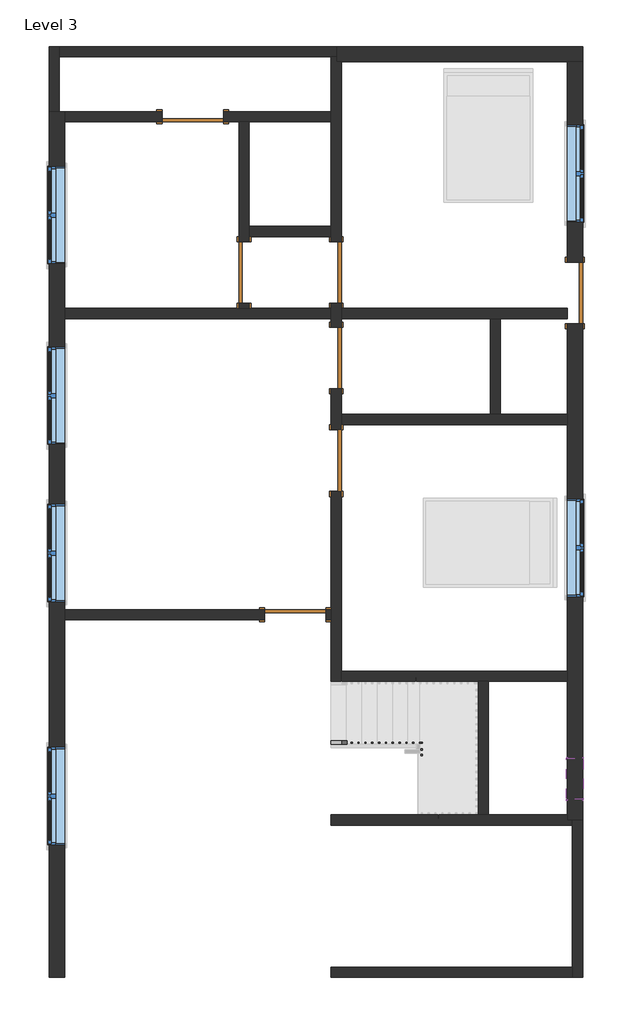
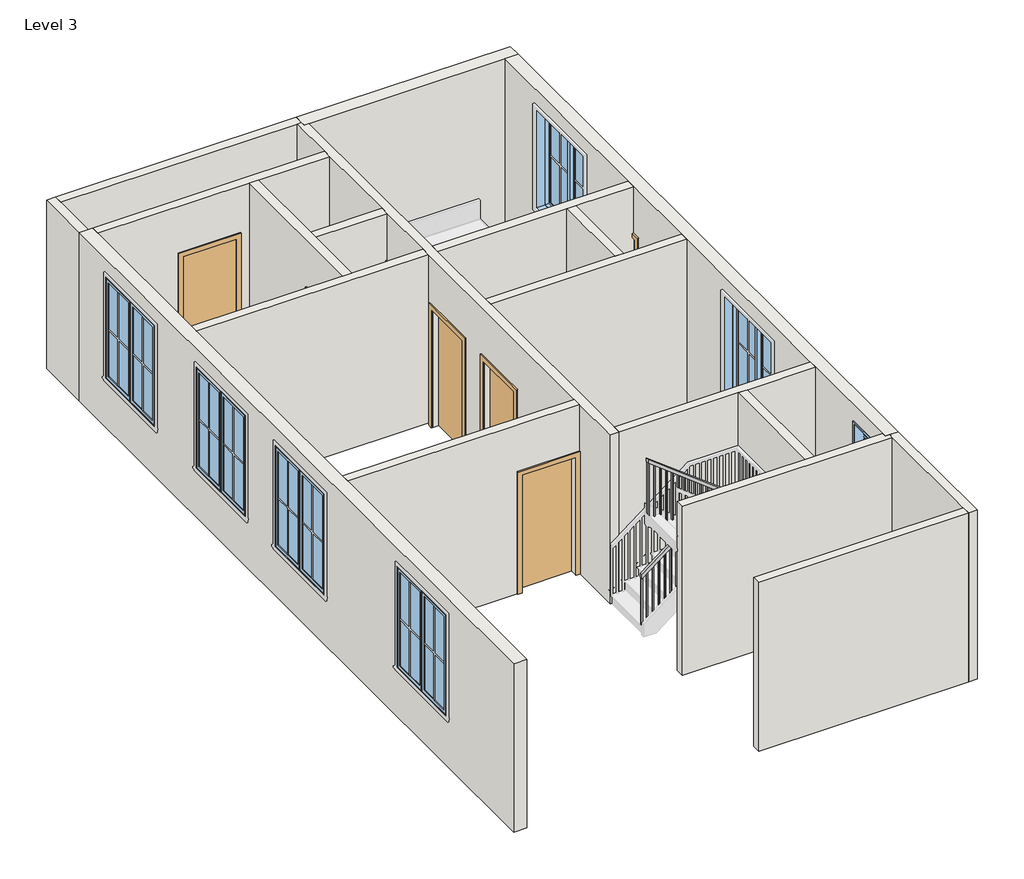
# One storey, part 1 of 2: 18 walls, 7 doors, 7 windows, 1 railing.
"""IFC4 building model written with IfcOpenShell, lengths in millimetres."""

from ifc_helpers import new_model, si_unit, frame, origin, place, context, project, spatial, polyline, outline, extrude, faceted_brep, transform, mapped, element, save
from components import door_686f89d2, door_16372e1c, door_0ca8825f, window_9ac97e1a, window_f2d8fef0

model = new_model("IFC4")

# Units and contexts
model_context = context("Model", 3, world=origin())
ifc_project = project(units=[si_unit("LENGTHUNIT", "METRE", prefix="MILLI")], contexts=[model_context])

# Site, building, storey
site = spatial("IfcSite", under=ifc_project)
building = spatial("IfcBuilding", under=site)
storey = spatial("IfcBuildingStorey", under=building, Name="Level 3", Elevation=3200.4)

# Doors
placement = place(None, origin())
door_shape = door_686f89d2(model_context)
element("IfcDoor", 1, ObjectType="Single-Flush : 36\" x 84\"", at=placement, inside=storey, context=model_context, shape_type="MappedRepresentation", body=[
    mapped(door_shape, transform((-2318.0415352, 3143.9226491, 3200.4), x_axis=(0.0, -1.0, 0.0), y_axis=(1.0, 0.0, 0.0), z_axis=(0.0, 0.0, 1.0))),
])
element("IfcDoor", 2, ObjectType="Single-Flush : 36\" x 84\"", at=placement, inside=storey, context=model_context, shape_type="MappedRepresentation", body=[
    mapped(door_shape, transform((-946.4415352, 3143.7222669, 3200.4), x_axis=(0.0, 1.0, 0.0), y_axis=(-1.0, 0.0, 0.0), z_axis=(0.0, 0.0, 1.0))),
])
element("IfcDoor", 3, ObjectType="Single-Flush : 36\" x 84\"", at=placement, inside=storey, context=model_context, shape_type="MappedRepresentation", body=[
    mapped(door_shape, transform((-946.4415352, 1874.1230313, 3200.4), x_axis=(0.0, 1.0, 0.0), y_axis=(-1.0, 0.0, 0.0), z_axis=(0.0, 0.0, 1.0))),
])
element("IfcDoor", 4, ObjectType="Single-Flush : 36\" x 84\"", at=placement, inside=storey, context=model_context, shape_type="MappedRepresentation", body=[
    mapped(door_shape, transform((-946.4415352, 350.1230313, 3200.4), x_axis=(0.0, 1.0, 0.0), y_axis=(-1.0, 0.0, 0.0), z_axis=(0.0, 0.0, 1.0))),
])
element("IfcDoor", 5, ObjectType="Single-Flush : 36\" x 84\"", at=placement, inside=storey, context=model_context, shape_type="MappedRepresentation", body=[
    mapped(door_shape, transform((-3080.0415352, 5453.9645078, 3200.4), x_axis=(1.0, 0.0, 0.0), y_axis=(0.0, 1.0, 0.0), z_axis=(0.0, 0.0, 1.0))),
])
door_2_shape = door_16372e1c(model_context)
element("IfcDoor", 6, ObjectType="Single-Flush : 36\" x 84\"", at=placement, inside=storey, context=model_context, shape_type="MappedRepresentation", body=[
    mapped(door_2_shape, transform((-1556.0415352, -1935.8769687, 3200.4), x_axis=(1.0, 0.0, 0.0), y_axis=(0.0, 1.0, 0.0), z_axis=(0.0, 0.0, 1.0))),
])
door_3_shape = door_0ca8825f(model_context)
element("IfcDoor", 7, ObjectType="Single-Flush : 36\" x 84\"", at=placement, inside=storey, context=model_context, shape_type="MappedRepresentation", body=[
    mapped(door_3_shape, transform((2596.8584648, 2839.3230313, 3200.4), x_axis=(0.0, -1.0, 0.0), y_axis=(1.0, 0.0, 0.0), z_axis=(0.0, 0.0, 1.0))),
])

# Railing
element("IfcRailing", 8, ObjectType="Handrail - Rectangular", at=placement, inside=storey, context=model_context, shape_type="SolidModel", body=[
    faceted_brep([(-1022.6415352, -3810.4539367, 4284.1333333), (-1022.6415352, -3810.4539367, 4219.9783974), (-1022.6415352, -3861.2539367, 4219.9783974), (-1022.6415352, -3861.2539367, 4284.1333333), (218.4221038, -3810.4539367, 5241.3605883), (269.2221038, -3810.4539367, 5216.3874824), (269.2221038, -3861.2539367, 5216.3874824), (218.4221038, -3861.2539367, 5241.3605883), (218.4221038, -3810.4539367, 5300.1333333), (269.2221038, -3810.4539367, 5249.3333333), (269.2221038, -3861.2539367, 5249.3333333), (218.4221038, -3861.2539367, 5300.1333333), (345.4221038, -3810.4539367, 5300.1333333), (345.4221038, -3810.4539367, 5249.3333333), (294.6221038, -3861.2539367, 5249.3333333), (294.6221038, -3861.2539367, 5300.1333333), (345.4221038, -3937.4539367, 5300.1333333), (345.4221038, -3937.4539367, 5249.3333333), (294.6221038, -3937.4539367, 5249.3333333), (294.6221038, -3937.4539367, 5300.1333333), (345.4221038, -3993.2769687, 5300.1333333), (294.6221038, -3993.2769687, 5300.1333333), (294.6221038, -4044.0769687, 5249.3333333), (345.4221038, -4044.0769687, 5249.3333333)], [[[0, 1, 2, 3]], [[1, 0, 4, 5]], [[2, 1, 5, 6]], [[3, 2, 6, 7]], [[0, 3, 7, 4]], [[5, 4, 8, 9]], [[6, 5, 9, 10]], [[7, 6, 10, 11]], [[4, 7, 11, 8]], [[9, 8, 12, 13]], [[10, 9, 13, 14]], [[11, 10, 14, 15]], [[8, 11, 15, 12]], [[13, 12, 16, 17]], [[14, 13, 17, 18]], [[15, 14, 18, 19]], [[12, 15, 19, 16]], [[20, 21, 22, 23]], [[17, 16, 20, 23]], [[18, 17, 23, 22]], [[19, 18, 22, 21]], [[16, 19, 21, 20]]]),
    faceted_brep([(345.4221038, -3993.2769687, 5300.1333333), (345.4221038, -4044.0769687, 5249.3333333), (294.6221038, -4044.0769687, 5249.3333333), (294.6221038, -3993.2769687, 5300.1333333), (345.4221038, -3993.2769687, 5430.2848366), (294.6221038, -3993.2769687, 5405.3117307), (294.6221038, -4044.0769687, 5405.3117307), (345.4221038, -4044.0769687, 5430.2848366)], [[[0, 1, 2, 3]], [[4, 5, 6, 7]], [[1, 0, 4, 7]], [[2, 1, 7, 6]], [[3, 2, 6, 5]], [[0, 3, 5, 4]]]),
    faceted_brep([(345.4221038, -4044.0769687, 5430.2848366), (294.6221038, -4044.0769687, 5405.3117307), (294.6221038, -3993.2769687, 5405.3117307), (345.4221038, -3993.2769687, 5430.2848366), (-1022.6415352, -4044.0769687, 6485.4666667), (-1022.6415352, -3993.2769687, 6485.4666667), (-1022.6415352, -3993.2769687, 6421.3117307), (-1022.6415352, -4044.0769687, 6421.3117307)], [[[0, 1, 2, 3]], [[4, 5, 6, 7]], [[1, 0, 4, 7]], [[2, 1, 7, 6]], [[3, 2, 6, 5]], [[0, 3, 5, 4]]]),
    extrude(outline(polyline([(6397.1018032, -991.2528962), (6411.7949894, -1010.3028962), (5401.7333333, -1010.3028962), (5401.7333333, -991.2528962), (6397.1018032, -991.2528962)])), frame((0.0, -4028.2019687, 0.0), z_axis=(0.0, 1.0, 0.0), x_axis=(0.0, 0.0, 1.0)), (0.0, 0.0, 1.0), 19.05),
    extrude(outline(polyline([(6318.7381431, -889.6528962), (6333.4313294, -908.7028962), (5401.7333333, -908.7028962), (5401.7333333, -889.6528962), (6318.7381431, -889.6528962)])), frame((0.0, -4028.2019687, 0.0), z_axis=(0.0, 1.0, 0.0), x_axis=(0.0, 0.0, 1.0)), (0.0, 0.0, 1.0), 19.05),
    extrude(outline(polyline([(6240.3744831, -788.0528962), (6255.0676694, -807.1028962), (5401.7333333, -807.1028962), (5401.7333333, -788.0528962), (6240.3744831, -788.0528962)])), frame((0.0, -4028.2019687, 0.0), z_axis=(0.0, 1.0, 0.0), x_axis=(0.0, 0.0, 1.0)), (0.0, 0.0, 1.0), 19.05),
    extrude(outline(polyline([(6162.0108231, -686.4528962), (6176.7040093, -705.5028962), (5232.4, -705.5028962), (5232.4, -686.4528962), (6162.0108231, -686.4528962)])), frame((0.0, -4028.2019687, 0.0), z_axis=(0.0, 1.0, 0.0), x_axis=(0.0, 0.0, 1.0)), (0.0, 0.0, 1.0), 19.05),
    extrude(outline(polyline([(6083.647163, -584.8528962), (6098.3403493, -603.9028962), (5232.4, -603.9028962), (5232.4, -584.8528962), (6083.647163, -584.8528962)])), frame((0.0, -4028.2019687, 0.0), z_axis=(0.0, 1.0, 0.0), x_axis=(0.0, 0.0, 1.0)), (0.0, 0.0, 1.0), 19.05),
    extrude(outline(polyline([(6005.283503, -483.2528962), (6019.9766892, -502.3028962), (5063.0666667, -502.3028962), (5063.0666667, -483.2528962), (6005.283503, -483.2528962)])), frame((0.0, -4028.2019687, 0.0), z_axis=(0.0, 1.0, 0.0), x_axis=(0.0, 0.0, 1.0)), (0.0, 0.0, 1.0), 19.05),
    extrude(outline(polyline([(5926.9198429, -381.6528962), (5941.6130292, -400.7028962), (5063.0666667, -400.7028962), (5063.0666667, -381.6528962), (5926.9198429, -381.6528962)])), frame((0.0, -4028.2019687, 0.0), z_axis=(0.0, 1.0, 0.0), x_axis=(0.0, 0.0, 1.0)), (0.0, 0.0, 1.0), 19.05),
    extrude(outline(polyline([(5848.5561829, -280.0528962), (5863.2493691, -299.1028962), (4893.7333333, -299.1028962), (4893.7333333, -280.0528962), (5848.5561829, -280.0528962)])), frame((0.0, -4028.2019687, 0.0), z_axis=(0.0, 1.0, 0.0), x_axis=(0.0, 0.0, 1.0)), (0.0, 0.0, 1.0), 19.05),
    extrude(outline(polyline([(5770.1925228, -178.4528962), (5784.8857091, -197.5028962), (4893.7333333, -197.5028962), (4893.7333333, -178.4528962), (5770.1925228, -178.4528962)])), frame((0.0, -4028.2019687, 0.0), z_axis=(0.0, 1.0, 0.0), x_axis=(0.0, 0.0, 1.0)), (0.0, 0.0, 1.0), 19.05),
    extrude(outline(polyline([(5691.8288628, -76.8528962), (5706.522049, -95.9028962), (4724.4, -95.9028962), (4724.4, -76.8528962), (5691.8288628, -76.8528962)])), frame((0.0, -4028.2019687, 0.0), z_axis=(0.0, 1.0, 0.0), x_axis=(0.0, 0.0, 1.0)), (0.0, 0.0, 1.0), 19.05),
    extrude(outline(polyline([(5613.4652027, 24.7471038), (5628.158389, 5.6971038), (4724.4, 5.6971038), (4724.4, 24.7471038), (5613.4652027, 24.7471038)])), frame((0.0, -4028.2019687, 0.0), z_axis=(0.0, 1.0, 0.0), x_axis=(0.0, 0.0, 1.0)), (0.0, 0.0, 1.0), 19.05),
    extrude(outline(polyline([(5535.1015427, 126.3471038), (5549.7947289, 107.2971038), (4724.4, 107.2971038), (4724.4, 126.3471038), (5535.1015427, 126.3471038)])), frame((0.0, -4028.2019687, 0.0), z_axis=(0.0, 1.0, 0.0), x_axis=(0.0, 0.0, 1.0)), (0.0, 0.0, 1.0), 19.05),
    extrude(outline(polyline([(5456.7378826, 227.9471038), (5471.4310689, 208.8971038), (4555.0666667, 208.8971038), (4555.0666667, 227.9471038), (5456.7378826, 227.9471038)])), frame((0.0, -4028.2019687, 0.0), z_axis=(0.0, 1.0, 0.0), x_axis=(0.0, 0.0, 1.0)), (0.0, 0.0, 1.0), 19.05),
    extrude(outline(polyline([(310.4971038, -3927.9289367), (329.5471038, -3927.9289367), (329.5471038, -3946.9789367), (310.4971038, -3946.9789367), (310.4971038, -3927.9289367)])), frame((0.0, 0.0, 4385.7333333), z_axis=(0.0, 0.0, 1.0), x_axis=(1.0, 0.0, 0.0)), (0.0, 0.0, 1.0), 863.6),
    extrude(outline(polyline([(288.6334648, -3845.3789367), (288.6334648, -3826.3289367), (307.6834648, -3826.3289367), (307.6834648, -3845.3789367), (288.6334648, -3845.3789367)])), frame((0.0, 0.0, 4385.7333333), z_axis=(0.0, 0.0, 1.0), x_axis=(1.0, 0.0, 0.0)), (0.0, 0.0, 1.0), 863.6),
    extrude(outline(polyline([(5167.6889111, 206.0834648), (5152.9957248, 187.0334648), (4216.4, 187.0334648), (4216.4, 206.0834648), (5167.6889111, 206.0834648)])), frame((0.0, -3845.3789367, 0.0), z_axis=(0.0, 1.0, 0.0), x_axis=(0.0, 0.0, 1.0)), (0.0, 0.0, 1.0), 19.05),
    extrude(outline(polyline([(5089.325251, 104.4834648), (5074.6320648, 85.4334648), (4047.0666667, 85.4334648), (4047.0666667, 104.4834648), (5089.325251, 104.4834648)])), frame((0.0, -3845.3789367, 0.0), z_axis=(0.0, 1.0, 0.0), x_axis=(0.0, 0.0, 1.0)), (0.0, 0.0, 1.0), 19.05),
    extrude(outline(polyline([(5010.961591, 2.8834648), (4996.2684047, -16.1665352), (4047.0666667, -16.1665352), (4047.0666667, 2.8834648), (5010.961591, 2.8834648)])), frame((0.0, -3845.3789367, 0.0), z_axis=(0.0, 1.0, 0.0), x_axis=(0.0, 0.0, 1.0)), (0.0, 0.0, 1.0), 19.05),
    extrude(outline(polyline([(4932.5979309, -98.7165352), (4917.9047447, -117.7665352), (4047.0666667, -117.7665352), (4047.0666667, -98.7165352), (4932.5979309, -98.7165352)])), frame((0.0, -3845.3789367, 0.0), z_axis=(0.0, 1.0, 0.0), x_axis=(0.0, 0.0, 1.0)), (0.0, 0.0, 1.0), 19.05),
    extrude(outline(polyline([(4854.2342709, -200.3165352), (4839.5410846, -219.3665352), (3877.7333333, -219.3665352), (3877.7333333, -200.3165352), (4854.2342709, -200.3165352)])), frame((0.0, -3845.3789367, 0.0), z_axis=(0.0, 1.0, 0.0), x_axis=(0.0, 0.0, 1.0)), (0.0, 0.0, 1.0), 19.05),
    extrude(outline(polyline([(4775.8706109, -301.9165352), (4761.1774246, -320.9665352), (3877.7333333, -320.9665352), (3877.7333333, -301.9165352), (4775.8706109, -301.9165352)])), frame((0.0, -3845.3789367, 0.0), z_axis=(0.0, 1.0, 0.0), x_axis=(0.0, 0.0, 1.0)), (0.0, 0.0, 1.0), 19.05),
    extrude(outline(polyline([(4697.5069508, -403.5165352), (4682.8137645, -422.5665352), (3708.4, -422.5665352), (3708.4, -403.5165352), (4697.5069508, -403.5165352)])), frame((0.0, -3845.3789367, 0.0), z_axis=(0.0, 1.0, 0.0), x_axis=(0.0, 0.0, 1.0)), (0.0, 0.0, 1.0), 19.05),
    extrude(outline(polyline([(4619.1432908, -505.1165352), (4604.4501045, -524.1665352), (3708.4, -524.1665352), (3708.4, -505.1165352), (4619.1432908, -505.1165352)])), frame((0.0, -3845.3789367, 0.0), z_axis=(0.0, 1.0, 0.0), x_axis=(0.0, 0.0, 1.0)), (0.0, 0.0, 1.0), 19.05),
    extrude(outline(polyline([(4540.7796307, -606.7165352), (4526.0864445, -625.7665352), (3539.0666667, -625.7665352), (3539.0666667, -606.7165352), (4540.7796307, -606.7165352)])), frame((0.0, -3845.3789367, 0.0), z_axis=(0.0, 1.0, 0.0), x_axis=(0.0, 0.0, 1.0)), (0.0, 0.0, 1.0), 19.05),
    extrude(outline(polyline([(4462.4159707, -708.3165352), (4447.7227844, -727.3665352), (3539.0666667, -727.3665352), (3539.0666667, -708.3165352), (4462.4159707, -708.3165352)])), frame((0.0, -3845.3789367, 0.0), z_axis=(0.0, 1.0, 0.0), x_axis=(0.0, 0.0, 1.0)), (0.0, 0.0, 1.0), 19.05),
    extrude(outline(polyline([(4384.0523106, -809.9165352), (4369.3591244, -828.9665352), (3369.7333333, -828.9665352), (3369.7333333, -809.9165352), (4384.0523106, -809.9165352)])), frame((0.0, -3845.3789367, 0.0), z_axis=(0.0, 1.0, 0.0), x_axis=(0.0, 0.0, 1.0)), (0.0, 0.0, 1.0), 19.05),
    extrude(outline(polyline([(4305.6886506, -911.5165352), (4290.9954643, -930.5665352), (3369.7333333, -930.5665352), (3369.7333333, -911.5165352), (4305.6886506, -911.5165352)])), frame((0.0, -3845.3789367, 0.0), z_axis=(0.0, 1.0, 0.0), x_axis=(0.0, 0.0, 1.0)), (0.0, 0.0, 1.0), 19.05),
    extrude(outline(polyline([(310.4971038, -4009.1519687), (329.5471038, -4009.1519687), (329.5471038, -4028.2019687), (310.4971038, -4028.2019687), (310.4971038, -4009.1519687)])), frame((0.0, 0.0, 4385.7333333), z_axis=(0.0, 0.0, 1.0), x_axis=(1.0, 0.0, 0.0)), (0.0, 0.0, 1.0), 863.6),
    extrude(outline(polyline([(310.4971038, -3845.3789367), (310.4971038, -3826.3289367), (329.5471038, -3826.3289367), (329.5471038, -3845.3789367), (310.4971038, -3845.3789367)])), frame((0.0, 0.0, 4385.7333333), z_axis=(0.0, 0.0, 1.0), x_axis=(1.0, 0.0, 0.0)), (0.0, 0.0, 1.0), 863.6),
    extrude(outline(polyline([(6406.6185445, -1003.5915352), (6421.3117307, -1022.6415352), (5401.7333333, -1022.6415352), (5401.7333333, -1003.5915352), (6406.6185445, -1003.5915352)])), frame((0.0, -4028.2019687, 0.0), z_axis=(0.0, 1.0, 0.0), x_axis=(0.0, 0.0, 1.0)), (0.0, 0.0, 1.0), 19.05),
    extrude(outline(polyline([(4234.6715837, -1003.5915352), (4219.9783974, -1022.6415352), (3369.7333333, -1022.6415352), (3369.7333333, -1003.5915352), (4234.6715837, -1003.5915352)])), frame((0.0, -3845.3789367, 0.0), z_axis=(0.0, 1.0, 0.0), x_axis=(0.0, 0.0, 1.0)), (0.0, 0.0, 1.0), 19.05),
])

# Walls
element("IfcWall", 9, ObjectType="WALL 6\"", at=placement, inside=storey, context=model_context, shape_type="Brep", body=[
    faceted_brep([(-5061.2415352, 5531.7230313, 3200.4), (-5061.2415352, 6344.5230313, 3200.4), (-5061.2415352, 6496.9230313, 3200.4), (-5061.2415352, 6496.9230313, 6248.4), (-5061.2415352, 6344.5230313, 6248.4), (-5061.2415352, 5531.7230313, 6248.4), (-5213.6415352, 5531.7230313, 3200.4), (-5213.6415352, 5531.7230313, 6248.4), (-5213.6415352, 6496.9230313, 6248.4), (-5213.6415352, 6496.9230313, 3200.4)], [[[0, 1, 2, 3, 4, 5]], [[6, 7, 8, 9]], [[2, 1, 0, 6, 9]], [[0, 5, 7, 6]], [[3, 2, 9, 8]], [[5, 4, 3, 8, 7]]]),
])
element("IfcWall", 10, ObjectType="WALL 6\"", at=placement, inside=storey, context=model_context, shape_type="Brep", body=[
    faceted_brep([(-5061.2415352, 6344.5230313, 3200.4), (-1022.6415352, 6344.5230313, 3200.4), (-946.4415352, 6344.5230313, 3200.4), (-946.4415352, 6344.5230313, 6248.4), (-1022.6415352, 6344.5230313, 6248.4), (-5061.2415352, 6344.5230313, 6248.4), (-5061.2415352, 6496.9230313, 3200.4), (-5061.2415352, 6496.9230313, 6248.4), (-946.4415352, 6496.9230313, 6248.4), (-946.4415352, 6496.9230313, 3200.4)], [[[0, 1, 2, 3, 4, 5]], [[6, 7, 8, 9]], [[2, 1, 0, 6, 9]], [[3, 2, 9, 8]], [[0, 5, 7, 6]], [[5, 4, 3, 8, 7]]]),
])
element("IfcWall", 11, ObjectType="WALL 6\"", at=placement, inside=storey, context=model_context, shape_type="Brep", body=[
    faceted_brep([(-1022.6415352, 1416.9230313, 3200.4), (-1022.6415352, 807.3230313, 3200.4), (-1022.6415352, 807.3230313, 5334.0), (-1022.6415352, -107.0769687, 5334.0), (-1022.6415352, -107.0769687, 3200.4), (-1022.6415352, -1859.6769687, 3200.4), (-1022.6415352, -2012.0769687, 3200.4), (-1022.6415352, -2926.4769687, 3200.4), (-1022.6415352, -2926.4769687, 6248.4), (-1022.6415352, -2012.0769687, 6248.4), (-1022.6415352, -1859.6769687, 6248.4), (-1022.6415352, 2458.3230313, 6248.4), (-1022.6415352, 2610.7230313, 6248.4), (-1022.6415352, 3677.1222669, 6248.4), (-1022.6415352, 3829.5222669, 6248.4), (-1022.6415352, 5377.7645078, 6248.4), (-1022.6415352, 5530.1645078, 6248.4), (-1022.6415352, 6344.5230313, 6248.4), (-1022.6415352, 6344.5230313, 3200.4), (-1022.6415352, 5530.1645078, 3200.4), (-1022.6415352, 5377.7645078, 3200.4), (-1022.6415352, 3829.5222669, 3200.4), (-1022.6415352, 3677.1222669, 3200.4), (-1022.6415352, 3600.9222669, 3200.4), (-1022.6415352, 3600.9222669, 5334.0), (-1022.6415352, 2686.5222669, 5334.0), (-1022.6415352, 2686.5222669, 3200.4), (-1022.6415352, 2610.7230313, 3200.4), (-1022.6415352, 2458.3230313, 3200.4), (-1022.6415352, 2331.3230313, 3200.4), (-1022.6415352, 2331.3230313, 5334.0), (-1022.6415352, 1416.9230313, 5334.0), (-870.2415352, 807.3230313, 5334.0), (-870.2415352, 807.3230313, 3200.4), (-870.2415352, 883.5230313, 3200.4), (-870.2415352, 1035.9230313, 3200.4), (-870.2415352, 1416.9230313, 3200.4), (-870.2415352, 1416.9230313, 5334.0), (-870.2415352, 2331.3230313, 5334.0), (-870.2415352, 2331.3230313, 3200.4), (-870.2415352, 2458.3230313, 3200.4), (-870.2415352, 2610.7230313, 3200.4), (-870.2415352, 2686.5222669, 3200.4), (-870.2415352, 2686.5222669, 5334.0), (-870.2415352, 3600.9222669, 5334.0), (-870.2415352, 3600.9222669, 3200.4), (-870.2415352, 6268.3230313, 3200.4), (-870.2415352, 6268.3230313, 6248.4), (-870.2415352, 2610.7230313, 6248.4), (-870.2415352, 2458.3230313, 6248.4), (-870.2415352, 1035.9230313, 6248.4), (-870.2415352, 883.5230313, 6248.4), (-870.2415352, -2774.0769687, 6248.4), (-870.2415352, -2926.4769687, 6248.4), (-870.2415352, -2926.4769687, 3200.4), (-870.2415352, -2774.0769687, 3200.4), (-870.2415352, -107.0769687, 3200.4), (-870.2415352, -107.0769687, 5334.0), (-946.4415352, 6344.5230313, 3200.4), (-946.4415352, 6268.3230313, 3200.4), (-946.4415352, 6344.5230313, 6248.4), (-946.4415352, 6268.3230313, 6248.4)], [[[0, 1, 2, 3, 4, 5, 6, 7, 8, 9, 10, 11, 12, 13, 14, 15, 16, 17, 18, 19, 20, 21, 22, 23, 24, 25, 26, 27, 28, 29, 30, 31]], [[32, 33, 34, 35, 36, 37, 38, 39, 40, 41, 42, 43, 44, 45, 46, 47, 48, 49, 50, 51, 52, 53, 54, 55, 56, 57]], [[46, 45, 23, 22, 21, 20, 19, 18, 58, 59]], [[42, 41, 40, 39, 29, 28, 27, 26]], [[56, 55, 54, 7, 6, 5, 4]], [[36, 35, 34, 33, 1, 0]], [[18, 17, 60, 58]], [[60, 61, 59, 58]], [[61, 47, 46, 59]], [[8, 7, 54, 53]], [[24, 23, 45, 44]], [[25, 24, 44, 43]], [[26, 25, 43, 42]], [[30, 29, 39, 38]], [[31, 30, 38, 37]], [[0, 31, 37, 36]], [[2, 1, 33, 32]], [[3, 2, 32, 57]], [[4, 3, 57, 56]], [[17, 16, 15, 14, 13, 12, 11, 10, 9, 8, 53, 52, 51, 50, 49, 48, 47, 61, 60]]]),
])
element("IfcWall", 12, ObjectType="WALL 6\"", at=placement, inside=storey, context=model_context, shape_type="Brep", body=[
    faceted_brep([(2482.5584648, -2774.0769687, 3200.4), (-870.2415352, -2774.0769687, 3200.4), (-870.2415352, -2774.0769687, 6248.4), (2482.5584648, -2774.0769687, 6248.4), (2482.5584648, -2926.4769687, 3200.4), (2482.5584648, -2926.4769687, 6248.4), (1314.1584648, -2926.4769687, 6248.4), (1161.7584648, -2926.4769687, 6248.4), (-870.2415352, -2926.4769687, 6248.4), (-870.2415352, -2926.4769687, 3200.4), (1161.7584648, -2926.4769687, 3200.4), (1314.1584648, -2926.4769687, 3200.4)], [[[0, 1, 2, 3]], [[4, 5, 6, 7, 8, 9, 10, 11]], [[1, 0, 4, 11, 10, 9]], [[2, 1, 9, 8]], [[0, 3, 5, 4]], [[3, 2, 8, 7, 6, 5]]]),
])
element("IfcWall", 13, ObjectType="WALL 6\"", at=placement, inside=storey, context=model_context, shape_type="Brep", body=[
    faceted_brep([(2558.7584648, -4983.8769687, 3200.4), (2558.7584648, -5060.0769687, 3200.4), (2558.7584648, -7168.2769687, 3200.4), (2558.7584648, -7320.6769687, 3200.4), (2558.7584648, -7320.6769687, 6248.4), (2558.7584648, -7168.2769687, 6248.4), (2558.7584648, -5060.0769687, 6248.4), (2558.7584648, -4983.8769687, 6248.4), (2711.1584648, -4983.8769687, 3200.4), (2711.1584648, -4983.8769687, 6248.4), (2711.1584648, -7320.6769687, 6248.4), (2711.1584648, -7320.6769687, 3200.4)], [[[0, 1, 2, 3, 4, 5, 6, 7]], [[8, 9, 10, 11]], [[3, 2, 1, 0, 8, 11]], [[0, 7, 9, 8]], [[4, 3, 11, 10]], [[7, 6, 5, 4, 10, 9]]]),
])
element("IfcWall", 14, ObjectType="WALL 6\"", at=placement, inside=storey, context=model_context, shape_type="SweptSolid", body=[
    extrude(outline(polyline([(-1022.6415352, -7168.2769687), (2558.7584648, -7168.2769687), (2558.7584648, -7320.6769687), (-1022.6415352, -7320.6769687), (-1022.6415352, -7168.2769687)])), frame((0.0, 0.0, 3200.4), z_axis=(0.0, 0.0, 1.0), x_axis=(1.0, 0.0, 0.0)), (0.0, 0.0, 1.0), 3048.0),
])
element("IfcWall", 15, ObjectType="WALL 6\"", at=placement, inside=storey, context=model_context, shape_type="Brep", body=[
    faceted_brep([(2482.5584648, -4907.6769687, 3200.4), (1314.1584648, -4907.6769687, 3200.4), (1161.7584648, -4907.6769687, 3200.4), (-1022.6415352, -4907.6769687, 3200.4), (-1022.6415352, -4907.6769687, 6248.4), (1161.7584648, -4907.6769687, 6248.4), (1314.1584648, -4907.6769687, 6248.4), (2482.5584648, -4907.6769687, 6248.4), (2558.7584648, -5060.0769687, 3200.4), (2558.7584648, -5060.0769687, 6248.4), (-1022.6415352, -5060.0769687, 6248.4), (-1022.6415352, -5060.0769687, 3200.4), (2482.5584648, -4983.8769687, 3200.4), (2558.7584648, -4983.8769687, 3200.4), (2482.5584648, -4983.8769687, 6248.4), (2558.7584648, -4983.8769687, 6248.4)], [[[0, 1, 2, 3, 4, 5, 6, 7]], [[8, 9, 10, 11]], [[3, 2, 1, 0, 12, 13, 8, 11]], [[4, 3, 11, 10]], [[0, 7, 14, 12]], [[14, 15, 13, 12]], [[15, 9, 8, 13]], [[7, 6, 5, 4, 10, 9, 15, 14]]]),
])
element("IfcWall", 16, ObjectType="WALL 6\"", at=placement, inside=storey, context=model_context, shape_type="SweptSolid", body=[
    extrude(outline(polyline([(1161.7584648, -4907.6769687), (1161.7584648, -2926.4769687), (1314.1584648, -2926.4769687), (1314.1584648, -4907.6769687), (1161.7584648, -4907.6769687)])), frame((0.0, 0.0, 3200.4), z_axis=(0.0, 0.0, 1.0), x_axis=(1.0, 0.0, 0.0)), (0.0, 0.0, 1.0), 3048.0),
])
element("IfcWall", 17, ObjectType="WALL 6\"", at=placement, inside=storey, context=model_context, shape_type="SweptSolid", body=[
    extrude(outline(polyline([(5334.0, -1098.8415352), (3200.4, -1098.8415352), (3200.4, -1022.6415352), (6248.4, -1022.6415352), (6248.4, -4985.0415352), (3200.4, -4985.0415352), (3200.4, -2013.2415352), (5334.0, -2013.2415352), (5334.0, -1098.8415352)])), frame((0.0, -2012.0769687, 0.0), z_axis=(0.0, 1.0, 0.0), x_axis=(0.0, 0.0, 1.0)), (0.0, 0.0, 1.0), 152.4),
])
element("IfcWall", 18, ObjectType="WALL 6\"", at=placement, inside=storey, context=model_context, shape_type="Brep", body=[
    faceted_brep([(2482.5584648, 2458.3230313, 3200.4), (2482.5584648, 2458.3230313, 6248.4), (1491.9584648, 2458.3230313, 6248.4), (1339.5584648, 2458.3230313, 6248.4), (-870.2415352, 2458.3230313, 6248.4), (-870.2415352, 2458.3230313, 3200.4), (1339.5584648, 2458.3230313, 3200.4), (1491.9584648, 2458.3230313, 3200.4), (2482.5584648, 2610.7230313, 6248.4), (2482.5584648, 2610.7230313, 3200.4), (-870.2415352, 2610.7230313, 3200.4), (-870.2415352, 2610.7230313, 6248.4)], [[[0, 1, 2, 3, 4, 5, 6, 7]], [[8, 9, 10, 11]], [[9, 0, 7, 6, 5, 10]], [[1, 0, 9, 8]], [[5, 4, 11, 10]], [[1, 8, 11, 4, 3, 2]]]),
    faceted_brep([(-4985.0415352, 2458.3230313, 6248.4), (-4985.0415352, 2458.3230313, 3200.4), (-1022.6415352, 2458.3230313, 3200.4), (-1022.6415352, 2458.3230313, 6248.4), (-4985.0415352, 2610.7230313, 3200.4), (-4985.0415352, 2610.7230313, 6248.4), (-2394.2415352, 2610.7230313, 6248.4), (-2241.8415352, 2610.7230313, 6248.4), (-1022.6415352, 2610.7230313, 6248.4), (-1022.6415352, 2610.7230313, 3200.4), (-2241.8415352, 2610.7230313, 3200.4), (-2394.2415352, 2610.7230313, 3200.4)], [[[0, 1, 2, 3]], [[4, 5, 6, 7, 8, 9, 10, 11]], [[1, 4, 11, 10, 9, 2]], [[1, 0, 5, 4]], [[3, 2, 9, 8]], [[5, 0, 3, 8, 7, 6]]]),
])
element("IfcWall", 19, ObjectType="WALL 6\"", at=placement, inside=storey, context=model_context, shape_type="Brep", body=[
    faceted_brep([(-2622.8415352, 5377.7645078, 5334.0), (-2622.8415352, 5377.7645078, 3200.4), (-2394.2415352, 5377.7645078, 3200.4), (-2241.8415352, 5377.7645078, 3200.4), (-1022.6415352, 5377.7645078, 3200.4), (-1022.6415352, 5377.7645078, 6248.4), (-2241.8415352, 5377.7645078, 6248.4), (-2394.2415352, 5377.7645078, 6248.4), (-4985.0415352, 5377.7645078, 6248.4), (-4985.0415352, 5377.7645078, 3200.4), (-3537.2415352, 5377.7645078, 3200.4), (-3537.2415352, 5377.7645078, 5334.0), (-1022.6415352, 5530.1645078, 3200.4), (-2622.8415352, 5530.1645078, 3200.4), (-2622.8415352, 5530.1645078, 5334.0), (-3537.2415352, 5530.1645078, 5334.0), (-3537.2415352, 5530.1645078, 3200.4), (-4985.0415352, 5530.1645078, 3200.4), (-4985.0415352, 5530.1645078, 6248.4), (-1022.6415352, 5530.1645078, 6248.4)], [[[0, 1, 2, 3, 4, 5, 6, 7, 8, 9, 10, 11]], [[12, 13, 14, 15, 16, 17, 18, 19]], [[10, 9, 17, 16]], [[4, 3, 2, 1, 13, 12]], [[9, 8, 18, 17]], [[5, 4, 12, 19]], [[14, 13, 1, 0]], [[15, 14, 0, 11]], [[16, 15, 11, 10]], [[8, 7, 6, 5, 19, 18]]]),
])
element("IfcWall", 20, ObjectType="WALL 6\"", at=placement, inside=storey, context=model_context, shape_type="Brep", body=[
    faceted_brep([(-2394.2415352, 2686.7226491, 5334.0), (-2394.2415352, 2686.7226491, 3200.4), (-2394.2415352, 2610.7230313, 3200.4), (-2394.2415352, 2610.7230313, 6248.4), (-2394.2415352, 5377.7645078, 6248.4), (-2394.2415352, 5377.7645078, 3200.4), (-2394.2415352, 3601.1226491, 3200.4), (-2394.2415352, 3601.1226491, 5334.0), (-2241.8415352, 2610.7230313, 3200.4), (-2241.8415352, 2686.7226491, 3200.4), (-2241.8415352, 2686.7226491, 5334.0), (-2241.8415352, 3601.1226491, 5334.0), (-2241.8415352, 3601.1226491, 3200.4), (-2241.8415352, 3677.1222669, 3200.4), (-2241.8415352, 3829.5222669, 3200.4), (-2241.8415352, 5377.7645078, 3200.4), (-2241.8415352, 5377.7645078, 6248.4), (-2241.8415352, 3829.5222669, 6248.4), (-2241.8415352, 3677.1222669, 6248.4), (-2241.8415352, 2610.7230313, 6248.4)], [[[0, 1, 2, 3, 4, 5, 6, 7]], [[8, 9, 10, 11, 12, 13, 14, 15, 16, 17, 18, 19]], [[6, 5, 15, 14, 13, 12]], [[2, 1, 9, 8]], [[3, 2, 8, 19]], [[5, 4, 16, 15]], [[10, 9, 1, 0]], [[11, 10, 0, 7]], [[12, 11, 7, 6]], [[4, 3, 19, 18, 17, 16]]]),
])
element("IfcWall", 21, ObjectType="WALL 6\"", at=placement, inside=storey, context=model_context, shape_type="SweptSolid", body=[
    extrude(outline(polyline([(-1022.6415352, 3677.1222669), (-2241.8415352, 3677.1222669), (-2241.8415352, 3829.5222669), (-1022.6415352, 3829.5222669), (-1022.6415352, 3677.1222669)])), frame((0.0, 0.0, 3200.4), z_axis=(0.0, 0.0, 1.0), x_axis=(1.0, 0.0, 0.0)), (0.0, 0.0, 1.0), 3048.0),
])
element("IfcWall", 22, ObjectType="WALL 6\"", at=placement, inside=storey, context=model_context, shape_type="Brep", body=[
    faceted_brep([(-870.2415352, 883.5230313, 3200.4), (2482.5584648, 883.5230313, 3200.4), (2482.5584648, 883.5230313, 6248.4), (-870.2415352, 883.5230313, 6248.4), (-870.2415352, 1035.9230313, 3200.4), (-870.2415352, 1035.9230313, 6248.4), (1339.5584648, 1035.9230313, 6248.4), (1491.9584648, 1035.9230313, 6248.4), (2482.5584648, 1035.9230313, 6248.4), (2482.5584648, 1035.9230313, 3200.4), (1491.9584648, 1035.9230313, 3200.4), (1339.5584648, 1035.9230313, 3200.4)], [[[0, 1, 2, 3]], [[4, 5, 6, 7, 8, 9, 10, 11]], [[1, 0, 4, 11, 10, 9]], [[2, 1, 9, 8]], [[0, 3, 5, 4]], [[3, 2, 8, 7, 6, 5]]]),
])
element("IfcWall", 23, ObjectType="WALL 6\"", at=placement, inside=storey, context=model_context, shape_type="SweptSolid", body=[
    extrude(outline(polyline([(1339.5584648, 1035.9230313), (1339.5584648, 2458.3230313), (1491.9584648, 2458.3230313), (1491.9584648, 1035.9230313), (1339.5584648, 1035.9230313)])), frame((0.0, 0.0, 3200.4), z_axis=(0.0, 0.0, 1.0), x_axis=(1.0, 0.0, 0.0)), (0.0, 0.0, 1.0), 3048.0),
])
element("IfcWall", 24, ObjectType="WALL 9\"", at=placement, inside=storey, context=model_context, shape_type="Brep", body=[
    faceted_brep([(-946.4415352, 6268.3230313, 3200.4), (-870.2415352, 6268.3230313, 3200.4), (2482.5584648, 6268.3230313, 3200.4), (2711.1584648, 6268.3230313, 3200.4), (2711.1584648, 6268.3230313, 6248.4), (2482.5584648, 6268.3230313, 6248.4), (-870.2415352, 6268.3230313, 6248.4), (-946.4415352, 6268.3230313, 6248.4), (-946.4415352, 6496.9230313, 3200.4), (-946.4415352, 6496.9230313, 6248.4), (2711.1584648, 6496.9230313, 6248.4), (2711.1584648, 6496.9230313, 3200.4), (-946.4415352, 6344.5230313, 3200.4), (-946.4415352, 6344.5230313, 6248.4)], [[[0, 1, 2, 3, 4, 5, 6, 7]], [[8, 9, 10, 11]], [[3, 2, 1, 0, 12, 8, 11]], [[0, 7, 13, 9, 8, 12]], [[4, 3, 11, 10]], [[7, 6, 5, 4, 10, 9, 13]]]),
])
element("IfcWall", 25, ObjectType="WALL 9\"", at=placement, inside=storey, context=model_context, shape_type="Brep", body=[
    faceted_brep([(2482.5584648, 2382.1230313, 5334.0), (2482.5584648, 2382.1230313, 3200.4), (2482.5584648, 1035.9230313, 3200.4), (2482.5584648, 883.5230313, 3200.4), (2482.5584648, -2774.0769687, 3200.4), (2482.5584648, -2926.4769687, 3200.4), (2482.5584648, -4907.6769687, 3200.4), (2482.5584648, -4983.8769687, 3200.4), (2482.5584648, -4983.8769687, 6248.4), (2482.5584648, -4907.6769687, 6248.4), (2482.5584648, -2926.4769687, 6248.4), (2482.5584648, -2774.0769687, 6248.4), (2482.5584648, 883.5230313, 6248.4), (2482.5584648, 1035.9230313, 6248.4), (2482.5584648, 2458.3230313, 6248.4), (2482.5584648, 2610.7230313, 6248.4), (2482.5584648, 6268.3230313, 6248.4), (2482.5584648, 6268.3230313, 3200.4), (2482.5584648, 3296.5230313, 3200.4), (2482.5584648, 3296.5230313, 5334.0), (2482.5584648, 3887.0730313, 5943.6), (2482.5584648, 3887.0730313, 4114.8), (2482.5584648, 5334.8730313, 4114.8), (2482.5584648, 5334.8730313, 5943.6), (2482.5584648, -1669.1769687, 5943.6), (2482.5584648, -1669.1769687, 4114.8), (2482.5584648, -221.3769687, 4114.8), (2482.5584648, -221.3769687, 5943.6), (2482.5584648, -4069.4769687, 5943.6), (2482.5584648, -4679.0769687, 5943.6), (2482.5584648, -4679.0769687, 5334.0), (2482.5584648, -4069.4769687, 5334.0), (2711.1584648, -4983.8769687, 3200.4), (2711.1584648, 2382.1230313, 3200.4), (2711.1584648, 2382.1230313, 5334.0), (2711.1584648, 3296.5230313, 5334.0), (2711.1584648, 3296.5230313, 3200.4), (2711.1584648, 6268.3230313, 3200.4), (2711.1584648, 6268.3230313, 6248.4), (2711.1584648, -4983.8769687, 6248.4), (2711.1584648, 3887.0730313, 5943.6), (2711.1584648, 5334.8730313, 5943.6), (2711.1584648, 5334.8730313, 4114.8), (2711.1584648, 3887.0730313, 4114.8), (2711.1584648, -1669.1769687, 5943.6), (2711.1584648, -221.3769687, 5943.6), (2711.1584648, -221.3769687, 4114.8), (2711.1584648, -1669.1769687, 4114.8), (2711.1584648, -4069.4769687, 5943.6), (2711.1584648, -4069.4769687, 5334.0), (2711.1584648, -4679.0769687, 5334.0), (2711.1584648, -4679.0769687, 5943.6), (2558.7584648, -4983.8769687, 3200.4), (2558.7584648, -4983.8769687, 6248.4)], [[[0, 1, 2, 3, 4, 5, 6, 7, 8, 9, 10, 11, 12, 13, 14, 15, 16, 17, 18, 19], [20, 21, 22, 23], [24, 25, 26, 27], [28, 29, 30, 31]], [[32, 33, 34, 35, 36, 37, 38, 39], [40, 41, 42, 43], [44, 45, 46, 47], [48, 49, 50, 51]], [[18, 17, 37, 36]], [[7, 6, 5, 4, 3, 2, 1, 33, 32, 52]], [[8, 7, 52, 32, 39, 53]], [[17, 16, 38, 37]], [[34, 33, 1, 0]], [[35, 34, 0, 19]], [[36, 35, 19, 18]], [[21, 20, 40, 43]], [[22, 21, 43, 42]], [[23, 22, 42, 41]], [[20, 23, 41, 40]], [[25, 24, 44, 47]], [[26, 25, 47, 46]], [[27, 26, 46, 45]], [[24, 27, 45, 44]], [[49, 48, 28, 31]], [[50, 49, 31, 30]], [[51, 50, 30, 29]], [[48, 51, 29, 28]], [[16, 15, 14, 13, 12, 11, 10, 9, 8, 53, 39, 38]]]),
])
element("IfcWall", 26, ObjectType="WALL 9\"", at=placement, inside=storey, context=model_context, shape_type="Brep", body=[
    faceted_brep([(-4985.0415352, -7320.6769687, 3200.4), (-4985.0415352, -2012.0769687, 3200.4), (-4985.0415352, -1859.6769687, 3200.4), (-4985.0415352, 2458.3230313, 3200.4), (-4985.0415352, 2610.7230313, 3200.4), (-4985.0415352, 5377.7645078, 3200.4), (-4985.0415352, 5530.1645078, 3200.4), (-4985.0415352, 5531.7230313, 3200.4), (-4985.0415352, 5531.7230313, 6248.4), (-4985.0415352, 5530.1645078, 6248.4), (-4985.0415352, 5377.7645078, 6248.4), (-4985.0415352, 2610.7230313, 6248.4), (-4985.0415352, 2458.3230313, 6248.4), (-4985.0415352, -1859.6769687, 6248.4), (-4985.0415352, -2012.0769687, 6248.4), (-4985.0415352, -7320.6769687, 6248.4), (-4985.0415352, 4718.1437696, 5943.6), (-4985.0415352, 4718.1437696, 4114.8), (-4985.0415352, 3270.3437696, 4114.8), (-4985.0415352, 3270.3437696, 5943.6), (-4985.0415352, 2039.2230313, 5943.6), (-4985.0415352, 2039.2230313, 4114.8), (-4985.0415352, 591.4230313, 4114.8), (-4985.0415352, 591.4230313, 5943.6), (-4985.0415352, -297.5769687, 5943.6), (-4985.0415352, -297.5769687, 4114.8), (-4985.0415352, -1745.3769687, 4114.8), (-4985.0415352, -1745.3769687, 5943.6), (-4985.0415352, -3904.3769687, 5943.6), (-4985.0415352, -3904.3769687, 4114.8), (-4985.0415352, -5352.1769687, 4114.8), (-4985.0415352, -5352.1769687, 5943.6), (-5213.6415352, -7320.6769687, 3200.4), (-5213.6415352, -7320.6769687, 6248.4), (-5213.6415352, 5531.7230313, 6248.4), (-5213.6415352, 5531.7230313, 3200.4), (-5213.6415352, 4718.1437696, 5943.6), (-5213.6415352, 3270.3437696, 5943.6), (-5213.6415352, 3270.3437696, 4114.8), (-5213.6415352, 4718.1437696, 4114.8), (-5213.6415352, 2039.2230313, 5943.6), (-5213.6415352, 591.4230313, 5943.6), (-5213.6415352, 591.4230313, 4114.8), (-5213.6415352, 2039.2230313, 4114.8), (-5213.6415352, -297.5769687, 5943.6), (-5213.6415352, -1745.3769687, 5943.6), (-5213.6415352, -1745.3769687, 4114.8), (-5213.6415352, -297.5769687, 4114.8), (-5213.6415352, -3904.3769687, 5943.6), (-5213.6415352, -5352.1769687, 5943.6), (-5213.6415352, -5352.1769687, 4114.8), (-5213.6415352, -3904.3769687, 4114.8), (-5061.2415352, 5531.7230313, 3200.4), (-5061.2415352, 5531.7230313, 6248.4)], [[[0, 1, 2, 3, 4, 5, 6, 7, 8, 9, 10, 11, 12, 13, 14, 15], [16, 17, 18, 19], [20, 21, 22, 23], [24, 25, 26, 27], [28, 29, 30, 31]], [[32, 33, 34, 35], [36, 37, 38, 39], [40, 41, 42, 43], [44, 45, 46, 47], [48, 49, 50, 51]], [[7, 6, 5, 4, 3, 2, 1, 0, 32, 35, 52]], [[8, 7, 52, 35, 34, 53]], [[0, 15, 33, 32]], [[17, 16, 36, 39]], [[18, 17, 39, 38]], [[19, 18, 38, 37]], [[16, 19, 37, 36]], [[21, 20, 40, 43]], [[22, 21, 43, 42]], [[23, 22, 42, 41]], [[20, 23, 41, 40]], [[25, 24, 44, 47]], [[26, 25, 47, 46]], [[27, 26, 46, 45]], [[24, 27, 45, 44]], [[29, 28, 48, 51]], [[30, 29, 51, 50]], [[31, 30, 50, 49]], [[28, 31, 49, 48]], [[15, 14, 13, 12, 11, 10, 9, 8, 53, 34, 33]]]),
])

# Windows
window_shape = window_9ac97e1a(model_context)
element("IfcWindow", 27, ObjectType="Window-Casement-Double : 57\" x 72\"", at=placement, inside=storey, context=model_context, shape_type="MappedRepresentation", body=[
    mapped(window_shape, transform((-5099.3415352, 3994.2437696, 3200.4), x_axis=(0.0, 1.0, 0.0), y_axis=(-1.0, 0.0, 0.0), z_axis=(0.0, 0.0, 1.0))),
])
element("IfcWindow", 28, ObjectType="Window-Casement-Double : 57\" x 72\"", at=placement, inside=storey, context=model_context, shape_type="MappedRepresentation", body=[
    mapped(window_shape, transform((2596.8584648, 4610.9730313, 3200.4), x_axis=(0.0, -1.0, 0.0), y_axis=(1.0, 0.0, 0.0), z_axis=(0.0, 0.0, 1.0))),
])
element("IfcWindow", 29, ObjectType="Window-Casement-Double : 57\" x 72\"", at=placement, inside=storey, context=model_context, shape_type="MappedRepresentation", body=[
    mapped(window_shape, transform((2596.8584648, -945.2769687, 3200.4), x_axis=(0.0, -1.0, 0.0), y_axis=(1.0, 0.0, 0.0), z_axis=(0.0, 0.0, 1.0))),
])
element("IfcWindow", 30, ObjectType="Window-Casement-Double : 57\" x 72\"", at=placement, inside=storey, context=model_context, shape_type="MappedRepresentation", body=[
    mapped(window_shape, transform((-5099.3415352, 1315.3230313, 3200.4), x_axis=(0.0, 1.0, 0.0), y_axis=(-1.0, 0.0, 0.0), z_axis=(0.0, 0.0, 1.0))),
])
element("IfcWindow", 31, ObjectType="Window-Casement-Double : 57\" x 72\"", at=placement, inside=storey, context=model_context, shape_type="MappedRepresentation", body=[
    mapped(window_shape, transform((-5099.3415352, -1021.4769687, 3200.4), x_axis=(0.0, 1.0, 0.0), y_axis=(-1.0, 0.0, 0.0), z_axis=(0.0, 0.0, 1.0))),
])
element("IfcWindow", 32, ObjectType="Window-Casement-Double : 57\" x 72\"", at=placement, inside=storey, context=model_context, shape_type="MappedRepresentation", body=[
    mapped(window_shape, transform((-5099.3415352, -4628.2769687, 3200.4), x_axis=(0.0, 1.0, 0.0), y_axis=(-1.0, 0.0, 0.0), z_axis=(0.0, 0.0, 1.0))),
])
window_2_shape = window_f2d8fef0(model_context)
element("IfcWindow", 33, ObjectType="Window-Louvers : 24\" x 24\"", at=placement, inside=storey, context=model_context, shape_type="MappedRepresentation", body=[
    mapped(window_2_shape, transform((2603.2084648, -4374.2769687, 4419.6), x_axis=(0.0, -1.0, 0.0), y_axis=(1.0, 0.0, 0.0), z_axis=(0.0, 0.0, 1.0))),
])

save(model, "model.ifc")

# Revit data of these elements
# Type "Single-Flush : 36\" x 84\""
#   Type Mark = "1"
#   Construction Type Id = "MDOOR"
#   Assembly Code = "C1020"
#   Analytic Construction = "Metal"
#   Thickness = 0' - 2"
#   Heat Transfer Coefficient (U) = 0.651978 BTU/(h·ft²·°F)
#   Height = 7' - 0"
#   Trim Projection Ext = 0' - 1"
#   Trim Projection Int = 0' - 1"
#   Trim Width = 0' - 3"
#   Width = 3' - 0"
#   Define Thermal Properties by = 1
#   Define Thermal Properties by = 1
#   Door Material = Door - Panel
#   Frame Material = Door - Frame
#   Visual Light Transmittance = 0
#   Solar Heat Gain Coefficient = 0
#   Function = (empty or 0)
#   Wall Closure = (empty or 0)
# Type "Handrail - Rectangular"
#   Assembly Code = "C2010400"
#   built-in parameter 1008612 = 0.0416667 (stored number, unit not read)
#   built-in parameter 1008611 = 0.0416667 (stored number, unit not read)
#   built-in parameter 1008609 = 0.333333 (stored number, unit not read)
#   built-in parameter 1008604 = 0.166667 (stored number, unit not read)
#   built-in parameter 1008603 = 0.166667 (stored number, unit not read)
#   Railing Height = 3' - 0"
#   built-in parameter 1008630 = 2
#   built-in parameter 1008610 = 2
#   built-in parameter 1008618 = Baluster - Square : 3/4"
# Type "WALL 6\""
#   Assembly Code = "B2010"
#   Layers, outside or top first: 0' - 6" no material (function 1)
# Type "WALL 9\""
#   Assembly Code = "B2010"
#   Layers, outside or top first: 0' - 9" no material (function 1)
# Type "Window-Casement-Double : 57\" x 72\""
#   Type Mark = "17"
#   Fire Rating = "0.5h"
#   Assembly Code = "B2020100"
#   Analytic Construction = "Double glazing - domestic"
#   Frame Extension [instance default] = 0' - 0 1/4"
#   Window Inset [instance default] = 0' - 0"
#   Wall Thickness [instance default] = 0' - 6"
#   Interior Wall Closure [instance default] = 0' - 2 1/4"
#   Half Width = 2' - 4 1/2"
#   Visual Light Transmittance = 0.81
#   Thermal Resistance (R) = 1.8146 (h·ft²·°F)/BTU
#   Solar Heat Gain Coefficient = 0.76
#   Rough Width = 4' - 9 1/2"
#   Rough Height = 6' - 0 1/2"
#   Height = 6' - 0"
#   Heat Transfer Coefficient (U) = 0.5511 BTU/(h·ft²·°F)
#   Exterior Wall Closure [instance default] = 0' - 1 1/4"
#   Extension Jamb [instance default] = 0' - 2 1/4"
#   Default Sill Height = 3' - 0"
#   Width = 4' - 9"
#   Define Thermal Properties by = 0
#   Muntin Visibility = yes
#   Interior Trim Visibility [instance default] = yes
#   Exterior Trim Visibility [instance default] = yes
#   Extension Jamb Visibility [instance default] = yes
#   Interior Trim Material = Wood - Stained
#   Muntin Pattern = Muntin Pattern_2x2 : Muntin Pattern_2x2
#   Interior Trim = Trim-Window-Interior-Flat : Picture Frame
#   Interior Frame Material = Wood - Stained
#   Glass Panel Material = Glass
#   Exterior Trim Material = Clad - White
#   Exterior Trim = Trim-Window-Exterior-Flat : with Sill
#   Exterior Frame Material = Clad - White
#   Wall Closure = (empty or 0)
# Type "Window-Louvers : 24\" x 24\""
#   Type Mark = "18"
#   Construction Type Id = "GSP4R"
#   Assembly Code = "B20"
#   Analytic Construction = "1/8 in Pilkington single glazing"
#   Visual Light Transmittance = 0.9
#   Thermal Resistance (R) = 1.53941 (h·ft²·°F)/BTU
#   Solar Heat Gain Coefficient = 0.78
#   Max Height = 1' - 11.74264"
#   Height = 2' - 0"
#   Heat Transfer Coefficient (U) = 0.6496 BTU/(h·ft²·°F)
#   Blade Width [instance default] = 1' - 10 1/2"
#   Blade Vertical Thickness = 0' - 0.35355"
#   Blade Thickness = 0' - 0 1/4"
#   Blade Spacing = 0' - 1 1/2"
#   Blade Height = 0' - 1.85355"
#   Blade Depth = 0' - 3"
#   Blade Angle = 45.00°
#   Default Sill Height = 3' - 0"
#   Trim Projection_Exterior = 0' - 0 1/2"
#   Trim Projection_Interior = 0' - 0 1/2"
#   Trim Width_Exterior = 0' - 1 1/2"
#   Trim Width_Interior = 0' - 1 1/2"
#   Width = 2' - 0"
#   Max Blade Count = 12
#   Define Thermal Properties by = 1
#   Blade Count = 12
#   Frame Material = Birch
#   Louver Material = Birch
#   Trim Exterior Material = Birch
#   Trim Interior Material = Birch
#   Wall Closure = (empty or 0)
# Elements 1, 2, 3, 4, 5, 6, 7 (IfcDoor, "Single-Flush : 36\" x 84\"")
#   Phase Created = New Construction
#   Materials on its faces: "Door - Frame", "Door - Panel"
# Element 8 (IfcRailing, "Handrail - Rectangular")
#   Phase Created = New Construction
# Elements 9, 10, 13, 14, 15, 17 (IfcWall, "WALL 6\"")
#   Top Offset = 0' - 0"
#   Base Offset = 0' - 0"
#   Unconnected Height = 10' - 0"
#   wall height = 10' - 0"
#   Phase Created = New Construction
#   Base Constraint = Level 3
#   Materials on its faces: "Default Wall", "Copper"
# Elements 11, 12, 16, 18, 19, 20, 21, 22, 23 (IfcWall, "WALL 6\"")
#   Top Offset = 0' - 0"
#   Base Offset = 0' - 0"
#   Unconnected Height = 10' - 0"
#   wall height = 10' - 0"
#   Phase Created = New Construction
#   Base Constraint = Level 3
#   Materials on its faces: "Default Wall"
# Elements 24, 25, 26 (IfcWall, "WALL 9\"")
#   Top Offset = 0' - 0"
#   Base Offset = 0' - 0"
#   Unconnected Height = 10' - 0"
#   wall height = 10' - 0"
#   Phase Created = New Construction
#   Base Constraint = Level 3
#   Materials on its faces: "Default Wall", "Copper"
# Element 27 (IfcWindow, "Window-Casement-Double : 57\" x 72\"")
#   Mark = "8"
#   Window Inset = 0' - 0"
#   Interior Wall Closure = 0' - 2 1/4"
#   Frame Extension = 0' - 0 1/4"
#   Exterior Wall Closure = 0' - 1 1/4"
#   Interior Trim Visibility = yes
#   Exterior Trim Visibility = yes
#   Phase Created = New Construction
#   Materials on its faces: "Wood - Stained", "Glass", "Clad - White"
# Element 28 (IfcWindow, "Window-Casement-Double : 57\" x 72\"")
#   Mark = "9"
#   Window Inset = 0' - 0"
#   Interior Wall Closure = 0' - 2 1/4"
#   Frame Extension = 0' - 0 1/4"
#   Exterior Wall Closure = 0' - 1 1/4"
#   Interior Trim Visibility = yes
#   Exterior Trim Visibility = yes
#   Phase Created = New Construction
#   Materials on its faces: "Wood - Stained", "Glass", "Clad - White"
# Element 29 (IfcWindow, "Window-Casement-Double : 57\" x 72\"")
#   Mark = "10"
#   Window Inset = 0' - 0"
#   Interior Wall Closure = 0' - 2 1/4"
#   Frame Extension = 0' - 0 1/4"
#   Exterior Wall Closure = 0' - 1 1/4"
#   Interior Trim Visibility = yes
#   Exterior Trim Visibility = yes
#   Phase Created = New Construction
#   Materials on its faces: "Wood - Stained", "Glass", "Clad - White"
# Element 30 (IfcWindow, "Window-Casement-Double : 57\" x 72\"")
#   Mark = "11"
#   Window Inset = 0' - 0"
#   Interior Wall Closure = 0' - 2 1/4"
#   Frame Extension = 0' - 0 1/4"
#   Exterior Wall Closure = 0' - 1 1/4"
#   Interior Trim Visibility = yes
#   Exterior Trim Visibility = yes
#   Phase Created = New Construction
#   Materials on its faces: "Wood - Stained", "Glass", "Clad - White"
# Element 31 (IfcWindow, "Window-Casement-Double : 57\" x 72\"")
#   Mark = "12"
#   Window Inset = 0' - 0"
#   Interior Wall Closure = 0' - 2 1/4"
#   Frame Extension = 0' - 0 1/4"
#   Exterior Wall Closure = 0' - 1 1/4"
#   Interior Trim Visibility = yes
#   Exterior Trim Visibility = yes
#   Phase Created = New Construction
#   Materials on its faces: "Wood - Stained", "Glass", "Clad - White"
# Element 32 (IfcWindow, "Window-Casement-Double : 57\" x 72\"")
#   Mark = "13"
#   Window Inset = 0' - 0"
#   Interior Wall Closure = 0' - 2 1/4"
#   Frame Extension = 0' - 0 1/4"
#   Exterior Wall Closure = 0' - 1 1/4"
#   Interior Trim Visibility = yes
#   Exterior Trim Visibility = yes
#   Phase Created = New Construction
#   Materials on its faces: "Wood - Stained", "Glass", "Clad - White"
# Element 33 (IfcWindow, "Window-Louvers : 24\" x 24\"")
#   Mark = "14"
#   Blade Width = 1' - 10 1/2"
#   Phase Created = New Construction
#   Materials on its faces: "Birch"
# Materials
#   "Door - Panel": class "Wood", colour RGB 210 159 95, transparency 0, Cost = 0
#   "Door - Frame": colour RGB 118 70 51, transparency 0, Cost = 0
#   "Wood - Stained": class "Wood", colour RGB 224 178 126, transparency 0, Cost = 0
#   "Glass": class "Glass", colour RGB 0 128 192, transparency 0.75, Description = "Soda Lime Glass", Cost = 0
#   "Clad - White": class "Wood", colour RGB 242 242 238, transparency 0, Cost = 0
#   "Birch": class "Wood", colour RGB 224 178 126, transparency 0, Description = "Betula Alleghaniensis", Cost = 0
#   "Default Wall": colour RGB 128 128 128, transparency 0, Cost = 0
#   "Copper": class "Metal", colour RGB 0 0 0, transparency 0, Description = "Copper, matte finish", Cost = 0
